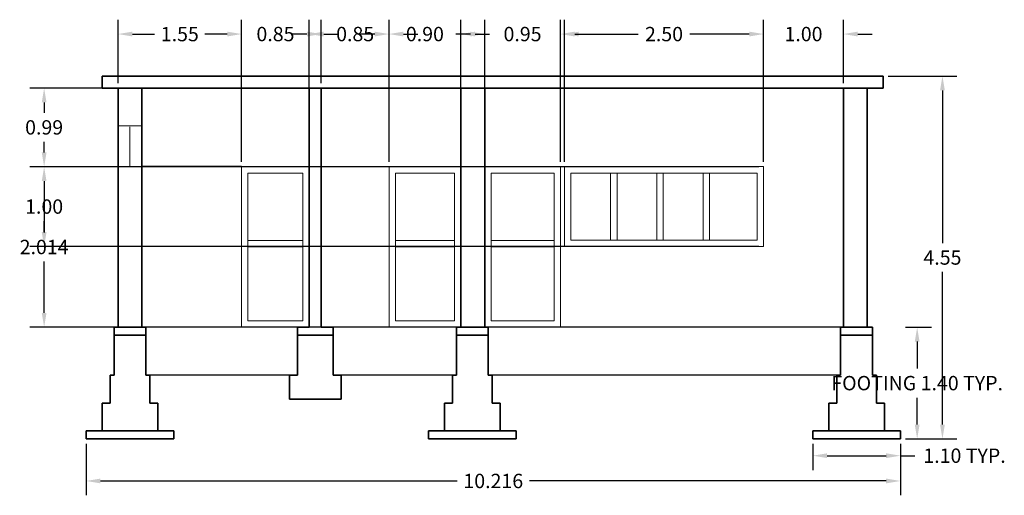
# Model space of a CAD drawing. Units: metres. Extents: x 37.9 to 70.9, y 22.7 to 44.8.
# Tile 4 of 4: x 58.6 to 70.9, y 38.6 to 44.6. Entities that reach past the tile are written whole.
import ezdxf

# ---------------------------------------------------------------- set-up
doc = ezdxf.new("R2010")
doc.units = ezdxf.units.M
doc.header["$LTSCALE"] = 50
doc.header["$MEASUREMENT"] = 0
doc.header["$PDMODE"] = 35
doc.header["$PDSIZE"] = -2
doc.linetypes.add('ACAD_ISO03W100', pattern=[30, 12, -18])
for name, color, linetype, lineweight in [('A-ANNO-DIMS', 2, 'Continuous', 18), ('A-SECT', 7, 'Continuous', 35), ('A-SECT-DOOR', 4, 'Continuous', 18), ('A-SECT-FLOR', 7, 'Continuous', 25), ('A-SECT-GLAZ', 4, 'Continuous', 18), ('A-SECT-ROOF', 7, 'Continuous', 35), ('S-FNDN', 7, 'Continuous', 35)]:
    doc.layers.add(name, color=color, linetype=linetype, lineweight=lineweight)
doc.styles.get("Standard").update_dxf_attribs({"font": 'arial.ttf'})
doc.dimstyles.get("Standard").update_dxf_attribs({"dimtxt": 0.18, "dimasz": 0.18, "dimexe": 0.18, "dimexo": 0.0625, "dimgap": 0.09, "dimtad": 0, "dimtih": 1, "dimtoh": 1, "dimzin": 0, "dimdsep": 46, "dimtxsty": 'Standard', "dimcen": 0.09, "dimadec": 0, "dimazin": 0, "dimtfac": 1, "dimtofl": 0, "dimtmove": 0, "dimatfit": 3, "dimfxl": 1, "dimtolj": 1, "dimtzin": 0, "dimarcsym": 0})

# ---------------------------------------------------------------- blocks, each defined once
blk = doc.blocks.new('FTG-STEPPED-1100-SECT')
for p, q in [((-0.15, 1.4), (-0.2, 1.4)), ((-0.2, 1.4), (-0.2, 0.8)), ((0.15, 1.4), (-0.15, 1.4)), ((0.15, 1.4), (0.2, 1.4)), ((0.2, 0.8), (0.2, 1.4)), ((0.2, 1.3), (-0.2, 1.3)), ((-0.2, 0.8), (-0.25, 0.8)), ((-0.25, 0.8), (-0.25, 0.45)), ((0.2, 0.8), (0.25, 0.8)), ((0.25, 0.8), (0.25, 0.45)), ((-0.25, 0.45), (-0.35, 0.45)), ((-0.35, 0.45), (-0.35, 0.1)), ((0.25, 0.45), (0.35, 0.45)), ((0.35, 0.45), (0.35, 0.1)), ((-0.35, 0.1), (-0.55, 0.1)), ((-0.55, 0.1), (-0.55, 0)), ((-0.55, 0), (0.55, 0)), ((-0.35, 0.1), (0.55, 0.1)), ((0.55, 0.1), (0.55, 0))]:
    blk.add_line(p, q)
blk = doc.blocks.new('*D19')
at = {"layer": 'A-ANNO-DIMS', "color": 0, "lineweight": -2, "transparency": 16777216}
for p, q in [((69.68, 40.713), (70.008, 40.713)), ((69.68, 39.313), (70.008, 39.313))]:
    blk.add_line(p, q, dxfattribs=at)
at = {"layer": 'A-ANNO-DIMS', "color": 0, "linetype": 'ACAD_ISO03W100', "lineweight": -2, "transparency": 16777216}
for p, q in [((69.828, 40.533), (69.828, 40.196)), ((69.828, 39.493), (69.828, 39.83))]:
    blk.add_line(p, q, dxfattribs=at)
at = {"layer": 'A-ANNO-DIMS', "color": 0, "transparency": 16777216}
for points in [[(69.798, 40.533), (69.858, 40.533), (69.828, 40.713)], [(69.798, 39.493), (69.858, 39.493), (69.828, 39.313)]]:
    blk.add_solid(points, dxfattribs=at)
at = {"layer": 'Defpoints', "color": 0, "transparency": 16777216}
for p in [(69.618, 40.713), (69.828, 40.713), (69.618, 39.313)]:
    blk.add_point(p, dxfattribs=at)
at = {"layer": 'A-ANNO-DIMS', "color": 0, "transparency": 16777216, "insert": (69.828, 40.013), "char_height": 0.18, "attachment_point": 5}
blk.add_mtext('\\A1;FOOTING 1.40 TYP.', dxfattribs=at)
blk = doc.blocks.new('*D20')
at = {"layer": 'A-ANNO-DIMS', "color": 0, "lineweight": -2, "transparency": 16777216}
for p, q in [((68.518, 39.251), (68.518, 38.923)), ((69.618, 39.251), (69.618, 38.923))]:
    blk.add_line(p, q, dxfattribs=at)
at = {"layer": 'A-ANNO-DIMS', "color": 0, "linetype": 'ACAD_ISO03W100', "lineweight": -2, "transparency": 16777216}
for p, q in [((68.698, 39.103), (69.438, 39.103)), ((69.618, 39.103), (69.798, 39.103))]:
    blk.add_line(p, q, dxfattribs=at)
at = {"layer": 'A-ANNO-DIMS', "color": 0, "transparency": 16777216}
for points in [[(68.698, 39.133), (68.698, 39.073), (68.518, 39.103)], [(69.438, 39.133), (69.438, 39.073), (69.618, 39.103)]]:
    blk.add_solid(points, dxfattribs=at)
at = {"layer": 'Defpoints', "color": 0, "transparency": 16777216}
for p in [(68.518, 39.313), (69.618, 39.313), (69.618, 39.103)]:
    blk.add_point(p, dxfattribs=at)
at = {"layer": 'A-ANNO-DIMS', "color": 0, "transparency": 16777216, "insert": (70.422, 39.103), "char_height": 0.18, "attachment_point": 5}
blk.add_mtext('\\A1;1.10 TYP.', dxfattribs=at)
blk = doc.blocks.new('*D42')
at = {"layer": 'A-ANNO-DIMS', "color": 0, "lineweight": -2, "transparency": 16777216}
for p, q in [((59.402, 39.251), (59.402, 38.606)), ((69.618, 39.251), (69.618, 38.606))]:
    blk.add_line(p, q, dxfattribs=at)
at = {"layer": 'A-ANNO-DIMS', "color": 0, "linetype": 'ACAD_ISO03W100', "lineweight": -2, "transparency": 16777216}
for p, q in [((59.582, 38.786), (64.055, 38.786)), ((69.438, 38.786), (64.965, 38.786))]:
    blk.add_line(p, q, dxfattribs=at)
at = {"layer": 'A-ANNO-DIMS', "color": 0, "transparency": 16777216}
for points in [[(59.582, 38.816), (59.582, 38.756), (59.402, 38.786)], [(69.438, 38.816), (69.438, 38.756), (69.618, 38.786)]]:
    blk.add_solid(points, dxfattribs=at)
at = {"layer": 'Defpoints', "color": 0, "transparency": 16777216}
for p in [(59.402, 39.313), (69.618, 39.313), (69.618, 38.786)]:
    blk.add_point(p, dxfattribs=at)
at = {"layer": 'A-ANNO-DIMS', "color": 0, "transparency": 16777216, "insert": (64.51, 38.786), "char_height": 0.18, "attachment_point": 5}
blk.add_mtext('\\A1;10.216', dxfattribs=at)
blk = doc.blocks.new('*D43')
at = {"layer": 'A-ANNO-DIMS', "color": 0, "lineweight": -2, "transparency": 16777216}
for p, q in [((69.465, 43.863), (70.325, 43.863)), ((69.68, 39.313), (70.325, 39.313))]:
    blk.add_line(p, q, dxfattribs=at)
at = {"layer": 'A-ANNO-DIMS', "color": 0, "linetype": 'ACAD_ISO03W100', "lineweight": -2, "transparency": 16777216}
for p, q in [((70.145, 43.683), (70.145, 41.77)), ((70.145, 39.493), (70.145, 41.407))]:
    blk.add_line(p, q, dxfattribs=at)
at = {"layer": 'A-ANNO-DIMS', "color": 0, "transparency": 16777216}
for points in [[(70.115, 43.683), (70.175, 43.683), (70.145, 43.863)], [(70.115, 39.493), (70.175, 39.493), (70.145, 39.313)]]:
    blk.add_solid(points, dxfattribs=at)
at = {"layer": 'Defpoints', "color": 0, "transparency": 16777216}
for p in [(69.402, 43.863), (70.145, 43.863), (69.618, 39.313)]:
    blk.add_point(p, dxfattribs=at)
at = {"layer": 'A-ANNO-DIMS', "color": 0, "transparency": 16777216, "insert": (70.145, 41.588), "char_height": 0.18, "attachment_point": 5}
blk.add_mtext('\\A1;4.55', dxfattribs=at)
blk = doc.blocks.new('*D44')
at = {"layer": 'A-ANNO-DIMS', "color": 0, "lineweight": -2, "transparency": 16777216}
for p, q in [((59.802, 43.776), (59.802, 44.57)), ((61.352, 42.79), (61.352, 44.57))]:
    blk.add_line(p, q, dxfattribs=at)
at = {"layer": 'A-ANNO-DIMS', "color": 0, "linetype": 'ACAD_ISO03W100', "lineweight": -2, "transparency": 16777216}
for p, q in [((59.982, 44.39), (60.261, 44.39)), ((61.172, 44.39), (60.893, 44.39))]:
    blk.add_line(p, q, dxfattribs=at)
at = {"layer": 'A-ANNO-DIMS', "color": 0, "transparency": 16777216}
for points in [[(59.982, 44.42), (59.982, 44.36), (59.802, 44.39)], [(61.172, 44.42), (61.172, 44.36), (61.352, 44.39)]]:
    blk.add_solid(points, dxfattribs=at)
at = {"layer": 'Defpoints', "color": 0, "transparency": 16777216}
for p in [(61.352, 44.39), (59.802, 43.713), (61.352, 42.727)]:
    blk.add_point(p, dxfattribs=at)
at = {"layer": 'A-ANNO-DIMS', "color": 0, "transparency": 16777216, "insert": (60.577, 44.39), "char_height": 0.18, "attachment_point": 5}
blk.add_mtext('\\A1;1.55', dxfattribs=at)
blk = doc.blocks.new('*D45')
at = {"layer": 'A-ANNO-DIMS', "color": 0, "lineweight": -2, "transparency": 16777216}
for p, q in [((61.352051, 42.789886), (61.352051, 44.570286)), ((62.202051, 42.789886), (62.202051, 44.570286))]:
    blk.add_line(p, q, dxfattribs=at)
at = {"layer": 'A-ANNO-DIMS', "color": 0, "linetype": 'ACAD_ISO03W100', "lineweight": -2, "transparency": 16777216}
for p, q in [((61.172051, 44.390286), (60.992051, 44.390286)), ((62.382051, 44.390286), (62.562051, 44.390286))]:
    blk.add_line(p, q, dxfattribs=at)
at = {"layer": 'A-ANNO-DIMS', "color": 0, "transparency": 16777216}
for points in [[(61.172051, 44.420286), (61.172051, 44.360286), (61.352051, 44.390286)], [(62.382051, 44.420286), (62.382051, 44.360286), (62.202051, 44.390286)]]:
    blk.add_solid(points, dxfattribs=at)
at = {"layer": 'Defpoints', "color": 0, "transparency": 16777216}
for p in [(62.202051, 44.390286), (61.352051, 42.727386), (62.202051, 42.727386)]:
    blk.add_point(p, dxfattribs=at)
at = {"layer": 'A-ANNO-DIMS', "color": 0, "transparency": 16777216, "insert": (61.777051, 44.390286), "char_height": 0.18, "attachment_point": 5}
blk.add_mtext('\\A1;0.85', dxfattribs=at)
blk = doc.blocks.new('*D46')
at = {"layer": 'A-ANNO-DIMS', "color": 0, "lineweight": -2, "transparency": 16777216}
for p, q in [((62.352051, 43.775786), (62.352051, 44.570286)), ((63.202051, 42.789886), (63.202051, 44.570286))]:
    blk.add_line(p, q, dxfattribs=at)
at = {"layer": 'A-ANNO-DIMS', "color": 0, "linetype": 'ACAD_ISO03W100', "lineweight": -2, "transparency": 16777216}
for p, q in [((62.172051, 44.390286), (61.992051, 44.390286)), ((63.382051, 44.390286), (63.562051, 44.390286))]:
    blk.add_line(p, q, dxfattribs=at)
at = {"layer": 'A-ANNO-DIMS', "color": 0, "transparency": 16777216}
for points in [[(62.172051, 44.420286), (62.172051, 44.360286), (62.352051, 44.390286)], [(63.382051, 44.420286), (63.382051, 44.360286), (63.202051, 44.390286)]]:
    blk.add_solid(points, dxfattribs=at)
at = {"layer": 'Defpoints', "color": 0, "transparency": 16777216}
for p in [(63.202051, 44.390286), (62.352051, 43.713286), (63.202051, 42.727386)]:
    blk.add_point(p, dxfattribs=at)
at = {"layer": 'A-ANNO-DIMS', "color": 0, "transparency": 16777216, "insert": (62.777051, 44.390286), "char_height": 0.18, "attachment_point": 5}
blk.add_mtext('\\A1;0.85', dxfattribs=at)
blk = doc.blocks.new('*D47')
at = {"layer": 'A-ANNO-DIMS', "color": 0, "lineweight": -2, "transparency": 16777216}
for p, q in [((63.202051, 42.789886), (63.202051, 44.570286)), ((64.102051, 42.789886), (64.102051, 44.570286))]:
    blk.add_line(p, q, dxfattribs=at)
at = {"layer": 'A-ANNO-DIMS', "color": 0, "linetype": 'ACAD_ISO03W100', "lineweight": -2, "transparency": 16777216}
for p, q in [((63.022051, 44.390286), (62.842051, 44.390286)), ((64.282051, 44.390286), (64.462051, 44.390286))]:
    blk.add_line(p, q, dxfattribs=at)
at = {"layer": 'A-ANNO-DIMS', "color": 0, "transparency": 16777216}
for points in [[(63.022051, 44.420286), (63.022051, 44.360286), (63.202051, 44.390286)], [(64.282051, 44.420286), (64.282051, 44.360286), (64.102051, 44.390286)]]:
    blk.add_solid(points, dxfattribs=at)
at = {"layer": 'Defpoints', "color": 0, "transparency": 16777216}
for p in [(64.102051, 44.390286), (63.202051, 42.727386), (64.102051, 42.727386)]:
    blk.add_point(p, dxfattribs=at)
at = {"layer": 'A-ANNO-DIMS', "color": 0, "transparency": 16777216, "insert": (63.652051, 44.390286), "char_height": 0.18, "attachment_point": 5}
blk.add_mtext('\\A1;0.90', dxfattribs=at)
blk = doc.blocks.new('*D48')
at = {"layer": 'A-ANNO-DIMS', "color": 0, "lineweight": -2, "transparency": 16777216}
for p, q in [((64.402051, 42.789886), (64.402051, 44.570286)), ((65.352051, 42.789886), (65.352051, 44.570286))]:
    blk.add_line(p, q, dxfattribs=at)
at = {"layer": 'A-ANNO-DIMS', "color": 0, "linetype": 'ACAD_ISO03W100', "lineweight": -2, "transparency": 16777216}
for p, q in [((64.222051, 44.390286), (64.042051, 44.390286)), ((65.532051, 44.390286), (65.712051, 44.390286))]:
    blk.add_line(p, q, dxfattribs=at)
at = {"layer": 'A-ANNO-DIMS', "color": 0, "transparency": 16777216}
for points in [[(64.222051, 44.420286), (64.222051, 44.360286), (64.402051, 44.390286)], [(65.532051, 44.420286), (65.532051, 44.360286), (65.352051, 44.390286)]]:
    blk.add_solid(points, dxfattribs=at)
at = {"layer": 'Defpoints', "color": 0, "transparency": 16777216}
for p in [(65.352051, 44.390286), (64.402051, 42.727386), (65.352051, 42.727386)]:
    blk.add_point(p, dxfattribs=at)
at = {"layer": 'A-ANNO-DIMS', "color": 0, "transparency": 16777216, "insert": (64.877051, 44.390286), "char_height": 0.18, "attachment_point": 5}
blk.add_mtext('\\A1;0.95', dxfattribs=at)
blk = doc.blocks.new('*D49')
at = {"layer": 'A-ANNO-DIMS', "color": 0, "lineweight": -2, "transparency": 16777216}
for p, q in [((65.402, 42.79), (65.402, 44.57)), ((67.902, 42.79), (67.902, 44.57))]:
    blk.add_line(p, q, dxfattribs=at)
at = {"layer": 'A-ANNO-DIMS', "color": 0, "linetype": 'ACAD_ISO03W100', "lineweight": -2, "transparency": 16777216}
for p, q in [((65.582, 44.39), (66.327, 44.39)), ((67.722, 44.39), (66.977, 44.39))]:
    blk.add_line(p, q, dxfattribs=at)
at = {"layer": 'A-ANNO-DIMS', "color": 0, "transparency": 16777216}
for points in [[(65.582, 44.42), (65.582, 44.36), (65.402, 44.39)], [(67.722, 44.42), (67.722, 44.36), (67.902, 44.39)]]:
    blk.add_solid(points, dxfattribs=at)
at = {"layer": 'Defpoints', "color": 0, "transparency": 16777216}
for p in [(67.902, 44.39), (65.402, 42.727), (67.902, 42.727)]:
    blk.add_point(p, dxfattribs=at)
at = {"layer": 'A-ANNO-DIMS', "color": 0, "transparency": 16777216, "insert": (66.652, 44.39), "char_height": 0.18, "attachment_point": 5}
blk.add_mtext('\\A1;2.50', dxfattribs=at)
blk = doc.blocks.new('*D50')
at = {"layer": 'A-ANNO-DIMS', "color": 0, "lineweight": -2, "transparency": 16777216}
for p, q in [((67.902051, 42.789886), (67.902051, 44.570286)), ((68.902051, 43.775786), (68.902051, 44.570286))]:
    blk.add_line(p, q, dxfattribs=at)
at = {"layer": 'A-ANNO-DIMS', "color": 0, "linetype": 'ACAD_ISO03W100', "lineweight": -2, "transparency": 16777216}
for p, q in [((67.722051, 44.390286), (67.542051, 44.390286)), ((69.082051, 44.390286), (69.262051, 44.390286))]:
    blk.add_line(p, q, dxfattribs=at)
at = {"layer": 'A-ANNO-DIMS', "color": 0, "transparency": 16777216}
for points in [[(67.722051, 44.420286), (67.722051, 44.360286), (67.902051, 44.390286)], [(69.082051, 44.420286), (69.082051, 44.360286), (68.902051, 44.390286)]]:
    blk.add_solid(points, dxfattribs=at)
at = {"layer": 'Defpoints', "color": 0, "transparency": 16777216}
for p in [(68.902051, 44.390286), (68.902051, 43.713286), (67.902051, 42.727386)]:
    blk.add_point(p, dxfattribs=at)
at = {"layer": 'A-ANNO-DIMS', "color": 0, "transparency": 16777216, "insert": (68.402051, 44.390286), "char_height": 0.18, "attachment_point": 5}
blk.add_mtext('\\A1;1.00', dxfattribs=at)
blk = doc.blocks.new('*D51')
at = {"layer": 'A-ANNO-DIMS', "color": 0, "lineweight": -2, "transparency": 16777216}
for p, q in [((59.74, 43.713), (58.695, 43.713)), ((61.29, 42.727), (58.695, 42.727))]:
    blk.add_line(p, q, dxfattribs=at)
at = {"layer": 'A-ANNO-DIMS', "color": 0, "linetype": 'ACAD_ISO03W100', "lineweight": -2, "transparency": 16777216}
for p, q in [((58.875, 43.533), (58.875, 43.402)), ((58.875, 42.907), (58.875, 43.038))]:
    blk.add_line(p, q, dxfattribs=at)
at = {"layer": 'A-ANNO-DIMS', "color": 0, "transparency": 16777216}
for points in [[(58.845, 43.533), (58.905, 43.533), (58.875, 43.713)], [(58.845, 42.907), (58.905, 42.907), (58.875, 42.727)]]:
    blk.add_solid(points, dxfattribs=at)
at = {"layer": 'Defpoints', "color": 0, "transparency": 16777216}
for p in [(59.802, 43.713), (58.875, 42.727), (61.352, 42.727)]:
    blk.add_point(p, dxfattribs=at)
at = {"layer": 'A-ANNO-DIMS', "color": 0, "transparency": 16777216, "insert": (58.875, 43.22), "char_height": 0.18, "attachment_point": 5}
blk.add_mtext('\\A1;0.99', dxfattribs=at)
blk = doc.blocks.new('*D52')
at = {"layer": 'A-ANNO-DIMS', "color": 0, "lineweight": -2, "transparency": 16777216}
for p, q in [((67.84, 42.727), (58.695, 42.727)), ((67.84, 41.727), (58.695, 41.727))]:
    blk.add_line(p, q, dxfattribs=at)
at = {"layer": 'A-ANNO-DIMS', "color": 0, "linetype": 'ACAD_ISO03W100', "lineweight": -2, "transparency": 16777216}
for p, q in [((58.875, 42.547), (58.875, 42.409)), ((58.875, 41.907), (58.875, 42.045))]:
    blk.add_line(p, q, dxfattribs=at)
at = {"layer": 'A-ANNO-DIMS', "color": 0, "transparency": 16777216}
for points in [[(58.845, 42.547), (58.905, 42.547), (58.875, 42.727)], [(58.845, 41.907), (58.905, 41.907), (58.875, 41.727)]]:
    blk.add_solid(points, dxfattribs=at)
at = {"layer": 'Defpoints', "color": 0, "transparency": 16777216}
for p in [(58.875, 42.727), (67.902, 42.727), (67.902, 41.727)]:
    blk.add_point(p, dxfattribs=at)
at = {"layer": 'A-ANNO-DIMS', "color": 0, "transparency": 16777216, "insert": (58.875, 42.227), "char_height": 0.18, "attachment_point": 5}
blk.add_mtext('\\A1;1.00', dxfattribs=at)
blk = doc.blocks.new('*D53')
at = {"layer": 'A-ANNO-DIMS', "color": 0, "lineweight": -2, "transparency": 16777216}
for p, q in [((61.29, 42.727), (58.695, 42.727)), ((61.29, 40.713), (58.695, 40.713))]:
    blk.add_line(p, q, dxfattribs=at)
at = {"layer": 'A-ANNO-DIMS', "color": 0, "linetype": 'ACAD_ISO03W100', "lineweight": -2, "transparency": 16777216}
for p, q in [((58.875, 42.547), (58.875, 41.902)), ((58.875, 40.893), (58.875, 41.538))]:
    blk.add_line(p, q, dxfattribs=at)
at = {"layer": 'A-ANNO-DIMS', "color": 0, "transparency": 16777216}
for points in [[(58.845, 42.547), (58.905, 42.547), (58.875, 42.727)], [(58.845, 40.893), (58.905, 40.893), (58.875, 40.713)]]:
    blk.add_solid(points, dxfattribs=at)
at = {"layer": 'Defpoints', "color": 0, "transparency": 16777216}
for p in [(61.352, 42.727), (58.875, 40.713), (61.352, 40.713)]:
    blk.add_point(p, dxfattribs=at)
at = {"layer": 'A-ANNO-DIMS', "color": 0, "transparency": 16777216, "insert": (58.875, 41.72), "char_height": 0.18, "attachment_point": 5}
blk.add_mtext('\\A1;2.014', dxfattribs=at)

msp = doc.modelspace()

# ---------------------------------------------------------------- linework, layer by layer
at = {"layer": 'A-SECT'}
for p, q in [((59.8021, 40.7133), (59.8021, 43.7133)), ((60.1021, 40.7133), (60.1021, 43.7133)), ((62.2021, 40.7133), (62.2021, 43.7133)), ((62.3521, 40.7133), (62.3521, 43.7133)), ((64.1021, 40.7133), (64.1021, 43.7133)), ((64.4021, 40.7133), (64.4021, 43.7133)), ((68.9021, 40.7133), (68.9021, 43.7133)), ((69.2021, 40.7133), (69.2021, 43.7133)), ((61.3521, 42.7274), (60.1021, 42.7274))]:
    msp.add_line(p, q, dxfattribs=at)
at = {"layer": 'A-SECT-DOOR'}
for p, q in [((61.3521, 40.7133), (61.3521, 42.7274)), ((63.2021, 40.7133), (63.2021, 42.7274)), ((63.2021, 42.7274), (64.1021, 42.7274)), ((64.4021, 42.7274), (65.3521, 42.7274)), ((65.3521, 40.7133), (65.3521, 42.7274)), ((62.1221, 41.8003), (61.4321, 41.8003)), ((64.0221, 41.8003), (63.2821, 41.8003)), ((65.2721, 41.8003), (64.4821, 41.8003)), ((62.1221, 41.7203), (61.4321, 41.7203)), ((64.0221, 41.7203), (63.2821, 41.7203)), ((65.2721, 41.7203), (64.4821, 41.7203))]:
    msp.add_line(p, q, dxfattribs=at)
for points in [[(61.3521, 40.7133), (62.2021, 40.7133), (62.2021, 42.7274), (61.3521, 42.7274)], [(61.3521, 40.7133), (62.2021, 40.7133), (62.2021, 42.7274), (61.3521, 42.7274)], [(61.4321, 40.7933), (62.1221, 40.7933), (62.1221, 42.6474), (61.4321, 42.6474)], [(63.2021, 40.7133), (64.1021, 40.7133), (64.1021, 42.7274), (63.2021, 42.7274)], [(63.2821, 40.7933), (64.0221, 40.7933), (64.0221, 42.6474), (63.2821, 42.6474)], [(64.4021, 40.7133), (65.3521, 40.7133), (65.3521, 42.7274), (64.4021, 42.7274)], [(64.4821, 40.7933), (65.2721, 40.7933), (65.2721, 42.6474), (64.4821, 42.6474)]]:
    msp.add_lwpolyline(points, close=True, dxfattribs=at)
at = {"layer": 'A-SECT-FLOR'}
for p, q in [((69.2021, 40.7133), (60.1521, 40.7133)), ((62.0521, 40.1133), (60.2021, 40.1133)), ((64.0472, 40.1133), (62.5021, 40.1133)), ((68.868, 40.1133), (64.4472, 40.1133)), ((69.3021, 40.1133), (69.268, 40.1133))]:
    msp.add_line(p, q, dxfattribs=at)
at = {"layer": 'A-SECT-GLAZ'}
for p, q in [((60.1021, 43.2394), (59.8021, 43.2394)), ((59.9521, 42.7274), (59.9521, 43.2274)), ((60.1021, 42.7274), (59.8021, 42.7274)), ((67.8221, 42.6474), (65.4821, 42.6474)), ((65.4821, 42.6474), (65.4821, 41.8074)), ((65.9821, 42.6474), (65.9821, 41.8074)), ((66.0621, 42.6474), (66.0621, 41.8074)), ((66.5621, 42.6474), (66.5621, 41.8074)), ((66.6421, 42.6474), (66.6421, 41.8074)), ((67.1421, 42.6474), (67.1421, 41.8074)), ((67.2221, 42.6474), (67.2221, 41.8074)), ((67.8221, 41.8074), (67.8221, 42.6474)), ((65.4821, 41.8074), (67.8221, 41.8074))]:
    msp.add_line(p, q, dxfattribs=at)
msp.add_lwpolyline([(65.4021, 41.7274), (67.9021, 41.7274), (67.9021, 42.7274), (65.4021, 42.7274)], close=True, dxfattribs=at)
at = {"layer": 'A-SECT-ROOF'}
for p, q in [((59.6021, 43.7133), (59.6021, 43.8633)), ((59.6021, 43.8633), (59.7021, 43.8633)), ((69.3021, 43.8633), (59.7021, 43.8633)), ((69.4021, 43.8633), (69.3021, 43.8633)), ((69.4021, 43.7133), (69.4021, 43.8633)), ((59.7021, 43.7133), (59.6021, 43.7133)), ((69.3021, 43.7133), (59.7021, 43.7133)), ((69.3021, 43.7133), (69.4021, 43.7133))]:
    msp.add_line(p, q, dxfattribs=at)
at = {"layer": 'S-FNDN'}
for p, q in [((60.1521, 40.7133), (60.1521, 40.6133)), ((62.2021, 40.7133), (62.0521, 40.7133)), ((62.0521, 40.7133), (62.0521, 40.6133)), ((62.3521, 40.7133), (62.5021, 40.7133)), ((62.5021, 40.7133), (62.5021, 40.6133)), ((62.0521, 40.6133), (62.5021, 40.6133)), ((62.0521, 40.6133), (62.0521, 40.1133)), ((62.5021, 40.6133), (62.5021, 40.1133)), ((62.0521, 40.1133), (61.9521, 40.1133)), ((61.9521, 40.1133), (61.9521, 39.8133)), ((62.5021, 40.1133), (62.6021, 40.1133)), ((62.6021, 40.1133), (62.6021, 39.9133)), ((62.6021, 39.8133), (62.6021, 39.9133)), ((61.9521, 39.8133), (62.6021, 39.8133))]:
    msp.add_line(p, q, dxfattribs=at)

# ---------------------------------------------------------------- block references
for p in [(59.9521, 39.3133), (64.2472, 39.3133), (69.068, 39.3133)]:
    msp.add_blockref('FTG-STEPPED-1100-SECT', p, dxfattribs=at)

# ---------------------------------------------------------------- dimensions: what is measured, and where the dimension line sits
at = {"layer": 'A-ANNO-DIMS'}
for base, p1, p2, override, picture, middle in [((61.3521, 44.3903), (59.8021, 43.7133), (61.3521, 42.7274), {"dimdec": 2, "dimlfac": 1, "dimrnd": 0, "dimzin": 0, "dimdsep": 46, "dimlunit": 2}, '*D44', (60.5771, 44.3903)), ((62.2021, 44.3903), (61.3521, 42.7274), (62.2021, 42.7274), {"dimdec": 2, "dimlfac": 1, "dimrnd": 0, "dimzin": 0, "dimdsep": 46, "dimlunit": 2}, '*D45', (61.7771, 44.3903)), ((63.2021, 44.3903), (62.3521, 43.7133), (63.2021, 42.7274), {"dimdec": 2, "dimlfac": 1, "dimrnd": 0, "dimzin": 0, "dimdsep": 46, "dimlunit": 2}, '*D46', (62.7771, 44.3903)), ((64.1021, 44.3903), (63.2021, 42.7274), (64.1021, 42.7274), {"dimdec": 2, "dimlfac": 1, "dimrnd": 0, "dimzin": 0, "dimdsep": 46, "dimlunit": 2}, '*D47', (63.6521, 44.3903)), ((65.3521, 44.3903), (64.4021, 42.7274), (65.3521, 42.7274), {"dimdec": 2, "dimlfac": 1, "dimrnd": 0, "dimzin": 0, "dimdsep": 46, "dimlunit": 2}, '*D48', (64.8771, 44.3903)), ((67.9021, 44.3903), (65.4021, 42.7274), (67.9021, 42.7274), {"dimdec": 2, "dimlfac": 1, "dimrnd": 0, "dimzin": 0, "dimdsep": 46, "dimlunit": 2}, '*D49', (66.6521, 44.3903)), ((68.9021, 44.3903), (67.9021, 42.7274), (68.9021, 43.7133), {"dimdec": 2, "dimlfac": 1, "dimrnd": 0, "dimzin": 0, "dimdsep": 46, "dimlunit": 2}, '*D50', (68.4021, 44.3903)), ((69.618, 38.7863), (59.4021, 39.3133), (69.618, 39.3133), {"dimdec": 3, "dimlfac": 1, "dimrnd": 0, "dimzin": 0, "dimdsep": 46, "dimlunit": 2}, '*D42', (64.51, 38.7863))]:
    dim = msp.add_linear_dim(base=base, p1=p1, p2=p2, dimstyle='Standard', override=override, dxfattribs=at)
    dim.commit()
    dim.dimension.update_dxf_attribs({"geometry": picture, "text_midpoint": middle})
for base, p1, p2, override, picture, middle in [((70.145, 43.8633), (69.618, 39.3133), (69.4021, 43.8633), {"dimdec": 2, "dimlfac": 1, "dimrnd": 0, "dimzin": 0, "dimdsep": 46, "dimlunit": 2}, '*D43', (70.145, 41.5883)), ((58.8751, 42.7274), (59.8021, 43.7133), (61.3521, 42.7274), {"dimdec": 2, "dimlfac": 1, "dimrnd": 0, "dimzin": 0, "dimdsep": 46, "dimlunit": 2}, '*D51', (58.8751, 43.2203)), ((58.8751, 40.7133), (61.3521, 42.7274), (61.3521, 40.7133), {"dimdec": 3, "dimlfac": 1, "dimrnd": 0, "dimzin": 0, "dimdsep": 46, "dimlunit": 2}, '*D53', (58.8751, 41.7203)), ((58.8751, 42.7274), (67.9021, 41.7274), (67.9021, 42.7274), {"dimdec": 2, "dimlfac": 1, "dimrnd": 0, "dimzin": 0, "dimdsep": 46, "dimlunit": 2}, '*D52', (58.8751, 42.2274))]:
    dim = msp.add_linear_dim(base=base, p1=p1, p2=p2, angle=90, dimstyle='Standard', override=override, dxfattribs=at)
    dim.commit()
    dim.dimension.update_dxf_attribs({"geometry": picture, "text_midpoint": middle})
dim = msp.add_linear_dim(base=(69.828, 40.7133), p1=(69.618, 39.3133), p2=(69.618, 40.7133), angle=90, text='FOOTING <> TYP.', dimstyle='Standard', override={"dimdec": 2, "dimlfac": 1, "dimrnd": 0, "dimzin": 0, "dimdsep": 46, "dimlunit": 2}, dxfattribs=at)
dim.commit()
dim.dimension.update_dxf_attribs({"geometry": '*D19', "text_midpoint": (69.828, 40.0133)})
dim = msp.add_linear_dim(base=(69.618, 39.1033), p1=(68.518, 39.3133), p2=(69.618, 39.3133), text='<> TYP.', dimstyle='Standard', override={"dimdec": 2, "dimlfac": 1, "dimrnd": 0, "dimzin": 0, "dimdsep": 46, "dimlunit": 2}, dxfattribs=at)
dim.commit()
dim.dimension.update_dxf_attribs({"geometry": '*D20', "text_midpoint": (70.4225, 39.1033)})

doc.saveas('drawing.dxf')
